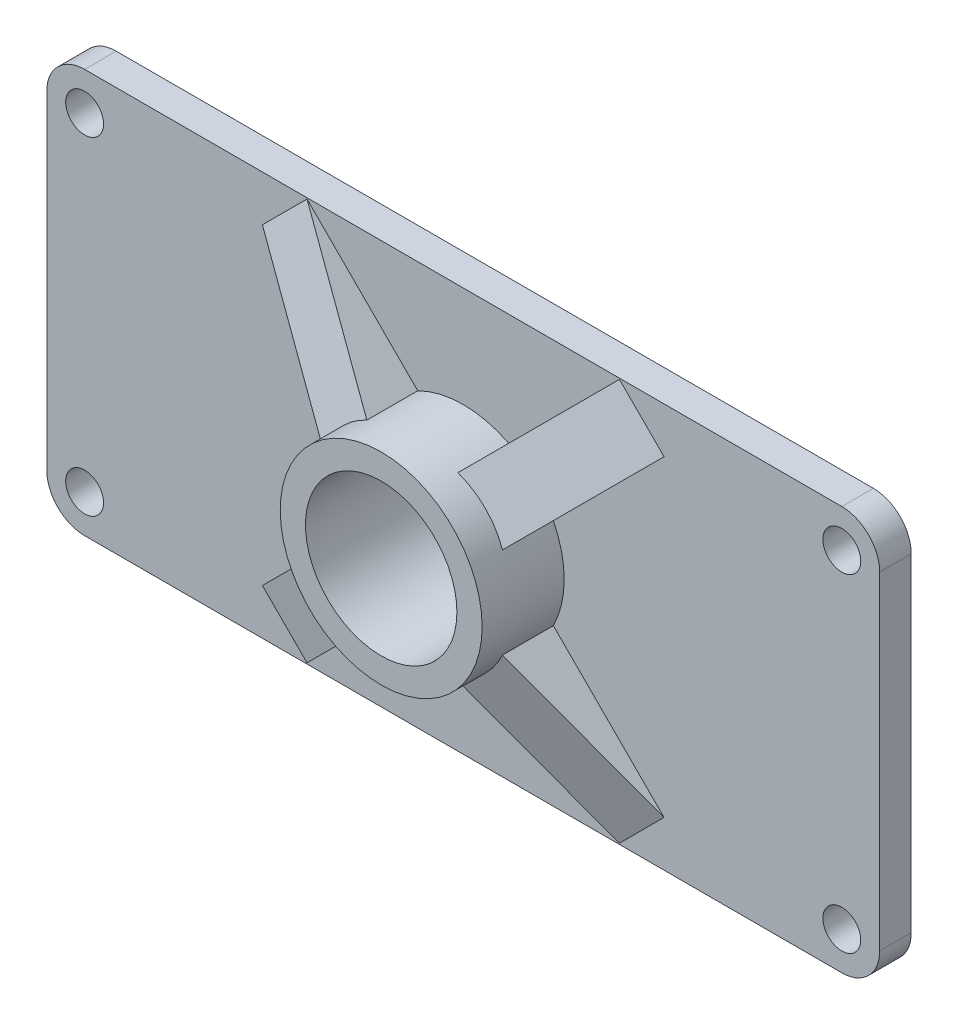
ISO-10303-21;
HEADER;
FILE_DESCRIPTION(('STEP AP214'),'2;1');
FILE_NAME('part.step','',(''),(''),'','','');
FILE_SCHEMA(('AUTOMOTIVE_DESIGN { 1 0 10303 214 1 1 1 1 }'));
ENDSEC;
DATA;
#1=APPLICATION_CONTEXT('core data for automotive mechanical design processes');
#2=APPLICATION_PROTOCOL_DEFINITION('international standard','automotive_design',2000,#1);
#3=PRODUCT_CONTEXT('',#1,'mechanical');
#4=PRODUCT('Part','Part','',(#3));
#5=PRODUCT_RELATED_PRODUCT_CATEGORY('part','',(#4));
#6=PRODUCT_DEFINITION_FORMATION('','',#4);
#7=PRODUCT_DEFINITION_CONTEXT('part definition',#1,'design');
#8=PRODUCT_DEFINITION('design','',#6,#7);
#9=PRODUCT_DEFINITION_SHAPE('','',#8);
#10=(LENGTH_UNIT() NAMED_UNIT(*) SI_UNIT(.MILLI.,.METRE.));
#11=(NAMED_UNIT(*) PLANE_ANGLE_UNIT() SI_UNIT($,.RADIAN.));
#12=(NAMED_UNIT(*) SI_UNIT($,.STERADIAN.) SOLID_ANGLE_UNIT());
#13=UNCERTAINTY_MEASURE_WITH_UNIT(LENGTH_MEASURE(1.E-05),#10,'distance_accuracy_value','');
#14=(GEOMETRIC_REPRESENTATION_CONTEXT(3) GLOBAL_UNCERTAINTY_ASSIGNED_CONTEXT((#13)) GLOBAL_UNIT_ASSIGNED_CONTEXT((#10,
#11,#12)) REPRESENTATION_CONTEXT('',''));
#15=CARTESIAN_POINT('',(0.,0.,0.));
#16=DIRECTION('',(0.,0.,1.));
#17=DIRECTION('',(1.,0.,0.));
#18=AXIS2_PLACEMENT_3D('',#15,#16,#17);
#19=CARTESIAN_POINT('',(-60.,-26.,5.));
#20=DIRECTION('',(0.,0.,1.));
#21=DIRECTION('',(1.,0.,0.));
#22=AXIS2_PLACEMENT_3D('',#19,#20,#21);
#23=PLANE('',#22);
#24=DIRECTION('',(0.70710678118655,-0.707106781186545,0.));
#25=VECTOR('',#24,1.);
#26=CARTESIAN_POINT('',(-13.4644660940675,20.5355339059328,5.));
#27=LINE('',#26,#25);
#28=CARTESIAN_POINT('',(14.2826265360351,-7.21155872416955,5.));
#29=VERTEX_POINT('',#28);
#30=CARTESIAN_POINT('',(31.8267955992102,-24.7557277873445,4.99999999999999));
#31=VERTEX_POINT('',#30);
#32=EDGE_CURVE('E225',#29,#31,#27,.T.);
#33=ORIENTED_EDGE('',*,*,#32,.T.);
#34=DIRECTION('',(-0.707106781186545,-0.70710678118655,0.));
#35=VECTOR('',#34,1.);
#36=CARTESIAN_POINT('',(-14.7087383067224,-71.2912616932773,5.));
#37=LINE('',#36,#35);
#38=CARTESIAN_POINT('',(24.7557277873447,-31.82679559921,5.));
#39=VERTEX_POINT('',#38);
#40=EDGE_CURVE('E228',#39,#31,#37,.F.);
#41=ORIENTED_EDGE('',*,*,#40,.F.);
#42=DIRECTION('',(0.70710678118655,-0.707106781186545,0.));
#43=VECTOR('',#42,1.);
#44=CARTESIAN_POINT('',(-20.5355339059329,13.4644660940673,5.));
#45=LINE('',#44,#43);
#46=CARTESIAN_POINT('',(7.21155872416964,-14.2826265360351,5.));
#47=VERTEX_POINT('',#46);
#48=EDGE_CURVE('E226',#47,#39,#45,.T.);
#49=ORIENTED_EDGE('',*,*,#48,.F.);
#50=CARTESIAN_POINT('',(0.,0.,5.));
#51=DIRECTION('',(0.,0.,1.));
#52=DIRECTION('',(1.,0.,0.));
#53=AXIS2_PLACEMENT_3D('',#50,#51,#52);
#54=CIRCLE('',#53,16.);
#55=CARTESIAN_POINT('',(-7.21155872416961,-14.2826265360351,5.));
#56=VERTEX_POINT('',#55);
#57=EDGE_CURVE('E251',#56,#47,#54,.T.);
#58=ORIENTED_EDGE('',*,*,#57,.F.);
#59=DIRECTION('',(-0.707106781186548,-0.707106781186547,0.));
#60=VECTOR('',#59,1.);
#61=CARTESIAN_POINT('',(-39.4644660940673,-46.5355339059327,5.));
#62=LINE('',#61,#60);
#63=CARTESIAN_POINT('',(-24.7557277873445,-31.82679559921,5.00000000000001));
#64=VERTEX_POINT('',#63);
#65=EDGE_CURVE('E237',#56,#64,#62,.T.);
#66=ORIENTED_EDGE('',*,*,#65,.T.);
#67=DIRECTION('',(-0.707106781186547,0.707106781186548,0.));
#68=VECTOR('',#67,1.);
#69=CARTESIAN_POINT('',(-45.2912616932773,-11.2912616932773,5.));
#70=LINE('',#69,#68);
#71=CARTESIAN_POINT('',(-31.82679559921,-24.7557277873445,5.));
#72=VERTEX_POINT('',#71);
#73=EDGE_CURVE('E242',#72,#64,#70,.F.);
#74=ORIENTED_EDGE('',*,*,#73,.F.);
#75=DIRECTION('',(-0.707106781186548,-0.707106781186547,0.));
#76=VECTOR('',#75,1.);
#77=CARTESIAN_POINT('',(-46.5355339059328,-39.4644660940673,5.));
#78=LINE('',#77,#76);
#79=CARTESIAN_POINT('',(-14.2826265360351,-7.21155872416961,5.));
#80=VERTEX_POINT('',#79);
#81=EDGE_CURVE('E238',#80,#72,#78,.T.);
#82=ORIENTED_EDGE('',*,*,#81,.F.);
#83=CARTESIAN_POINT('',(-14.2826265360352,7.21155872416946,5.));
#84=VERTEX_POINT('',#83);
#85=EDGE_CURVE('E256',#84,#80,#54,.T.);
#86=ORIENTED_EDGE('',*,*,#85,.F.);
#87=DIRECTION('',(-0.707106781186555,0.70710678118654,0.));
#88=VECTOR('',#87,1.);
#89=CARTESIAN_POINT('',(-20.5355339059333,13.4644660940675,5.));
#90=LINE('',#89,#88);
#91=CARTESIAN_POINT('',(-31.8267955992102,24.7557277873442,5.00000000000001));
#92=VERTEX_POINT('',#91);
#93=EDGE_CURVE('E56',#84,#92,#90,.T.);
#94=ORIENTED_EDGE('',*,*,#93,.T.);
#95=DIRECTION('',(0.70710678118654,0.707106781186555,0.));
#96=VECTOR('',#95,1.);
#97=CARTESIAN_POINT('',(-71.291261693277,-14.7087383067233,5.));
#98=LINE('',#97,#96);
#99=CARTESIAN_POINT('',(-24.7557277873449,31.8267955992098,4.99999999999999));
#100=VERTEX_POINT('',#99);
#101=EDGE_CURVE('E53',#100,#92,#98,.F.);
#102=ORIENTED_EDGE('',*,*,#101,.F.);
#103=DIRECTION('',(-0.707106781186555,0.70710678118654,0.));
#104=VECTOR('',#103,1.);
#105=CARTESIAN_POINT('',(-13.4644660940679,20.535533905933,5.));
#106=LINE('',#105,#104);
#107=CARTESIAN_POINT('',(-7.21155872416975,14.282626536035,5.));
#108=VERTEX_POINT('',#107);
#109=EDGE_CURVE('E187',#108,#100,#106,.T.);
#110=ORIENTED_EDGE('',*,*,#109,.F.);
#111=CARTESIAN_POINT('',(7.2115587241696,14.2826265360351,5.));
#112=VERTEX_POINT('',#111);
#113=EDGE_CURVE('E670',#112,#108,#54,.T.);
#114=ORIENTED_EDGE('',*,*,#113,.F.);
#115=DIRECTION('',(0.707106781186548,0.707106781186547,0.));
#116=VECTOR('',#115,1.);
#117=CARTESIAN_POINT('',(-46.5355339059328,-39.4644660940673,5.));
#118=LINE('',#117,#116);
#119=CARTESIAN_POINT('',(24.7557277873446,31.8267955992101,4.99999999999999));
#120=VERTEX_POINT('',#119);
#121=EDGE_CURVE('E211',#112,#120,#118,.T.);
#122=ORIENTED_EDGE('',*,*,#121,.T.);
#123=DIRECTION('',(0.707106781186547,-0.707106781186548,0.));
#124=VECTOR('',#123,1.);
#125=CARTESIAN_POINT('',(11.2912616932773,45.2912616932773,5.));
#126=LINE('',#125,#124);
#127=CARTESIAN_POINT('',(31.82679559921,24.7557277873446,5.));
#128=VERTEX_POINT('',#127);
#129=EDGE_CURVE('E213',#128,#120,#126,.F.);
#130=ORIENTED_EDGE('',*,*,#129,.F.);
#131=DIRECTION('',(0.707106781186548,0.707106781186547,0.));
#132=VECTOR('',#131,1.);
#133=CARTESIAN_POINT('',(-39.4644660940673,-46.5355339059327,5.));
#134=LINE('',#133,#132);
#135=CARTESIAN_POINT('',(14.2826265360351,7.21155872416959,5.));
#136=VERTEX_POINT('',#135);
#137=EDGE_CURVE('E206',#136,#128,#134,.T.);
#138=ORIENTED_EDGE('',*,*,#137,.F.);
#139=EDGE_CURVE('E260',#29,#136,#54,.T.);
#140=ORIENTED_EDGE('',*,*,#139,.F.);
#141=EDGE_LOOP('',(#33,#41,#49,#58,#66,#74,#82,#86,#94,#102,#110,#114,#122,#130,#138,#140));
#142=FACE_BOUND('',#141,.T.);
#143=DIRECTION('',(1.,0.,0.));
#144=VECTOR('',#143,1.);
#145=CARTESIAN_POINT('',(-60.,-32.,5.));
#146=LINE('',#145,#144);
#147=CARTESIAN_POINT('',(-60.,-32.,5.));
#148=VERTEX_POINT('',#147);
#149=CARTESIAN_POINT('',(60.,-32.,5.));
#150=VERTEX_POINT('',#149);
#151=EDGE_CURVE('E289',#148,#150,#146,.T.);
#152=ORIENTED_EDGE('',*,*,#151,.T.);
#153=CARTESIAN_POINT('',(60.,-26.,5.));
#154=DIRECTION('',(0.,0.,1.));
#155=DIRECTION('',(1.,0.,0.));
#156=AXIS2_PLACEMENT_3D('',#153,#154,#155);
#157=CIRCLE('',#156,6.);
#158=CARTESIAN_POINT('',(66.,-26.,5.));
#159=VERTEX_POINT('',#158);
#160=EDGE_CURVE('E295',#150,#159,#157,.T.);
#161=ORIENTED_EDGE('',*,*,#160,.T.);
#162=DIRECTION('',(0.,1.,0.));
#163=VECTOR('',#162,1.);
#164=CARTESIAN_POINT('',(66.,-26.,5.));
#165=LINE('',#164,#163);
#166=CARTESIAN_POINT('',(66.,26.,5.));
#167=VERTEX_POINT('',#166);
#168=EDGE_CURVE('E294',#159,#167,#165,.T.);
#169=ORIENTED_EDGE('',*,*,#168,.T.);
#170=CARTESIAN_POINT('',(60.,26.,5.));
#171=DIRECTION('',(0.,0.,1.));
#172=DIRECTION('',(-1.,0.,0.));
#173=AXIS2_PLACEMENT_3D('',#170,#171,#172);
#174=CIRCLE('',#173,6.);
#175=CARTESIAN_POINT('',(60.,32.,5.));
#176=VERTEX_POINT('',#175);
#177=EDGE_CURVE('E296',#167,#176,#174,.T.);
#178=ORIENTED_EDGE('',*,*,#177,.T.);
#179=DIRECTION('',(-1.,0.,0.));
#180=VECTOR('',#179,1.);
#181=CARTESIAN_POINT('',(-60.,32.,5.));
#182=LINE('',#181,#180);
#183=CARTESIAN_POINT('',(-60.,32.,5.));
#184=VERTEX_POINT('',#183);
#185=EDGE_CURVE('E297',#176,#184,#182,.T.);
#186=ORIENTED_EDGE('',*,*,#185,.T.);
#187=CARTESIAN_POINT('',(-60.,26.,5.));
#188=DIRECTION('',(0.,0.,1.));
#189=DIRECTION('',(-1.,0.,0.));
#190=AXIS2_PLACEMENT_3D('',#187,#188,#189);
#191=CIRCLE('',#190,6.);
#192=CARTESIAN_POINT('',(-66.,26.,5.));
#193=VERTEX_POINT('',#192);
#194=EDGE_CURVE('E299',#184,#193,#191,.T.);
#195=ORIENTED_EDGE('',*,*,#194,.T.);
#196=DIRECTION('',(0.,-1.,0.));
#197=VECTOR('',#196,1.);
#198=CARTESIAN_POINT('',(-66.,-26.,5.));
#199=LINE('',#198,#197);
#200=CARTESIAN_POINT('',(-66.,-26.,5.));
#201=VERTEX_POINT('',#200);
#202=EDGE_CURVE('E305',#193,#201,#199,.T.);
#203=ORIENTED_EDGE('',*,*,#202,.T.);
#204=CARTESIAN_POINT('',(-60.,-26.,5.));
#205=DIRECTION('',(0.,0.,1.));
#206=DIRECTION('',(1.,0.,0.));
#207=AXIS2_PLACEMENT_3D('',#204,#205,#206);
#208=CIRCLE('',#207,6.);
#209=EDGE_CURVE('E287',#201,#148,#208,.T.);
#210=ORIENTED_EDGE('',*,*,#209,.T.);
#211=EDGE_LOOP('',(#152,#161,#169,#178,#186,#195,#203,#210));
#212=FACE_BOUND('',#211,.T.);
#213=CARTESIAN_POINT('',(-60.,-26.,5.));
#214=DIRECTION('',(0.,0.,1.));
#215=DIRECTION('',(1.,0.,0.));
#216=AXIS2_PLACEMENT_3D('',#213,#214,#215);
#217=CIRCLE('',#216,3.);
#218=CARTESIAN_POINT('',(-57.,-26.,5.));
#219=VERTEX_POINT('',#218);
#220=EDGE_CURVE('E265',#219,#219,#217,.T.);
#221=ORIENTED_EDGE('',*,*,#220,.F.);
#222=EDGE_LOOP('',(#221));
#223=FACE_BOUND('',#222,.T.);
#224=CARTESIAN_POINT('',(60.,26.,5.));
#225=DIRECTION('',(0.,0.,1.));
#226=DIRECTION('',(1.,0.,0.));
#227=AXIS2_PLACEMENT_3D('',#224,#225,#226);
#228=CIRCLE('',#227,3.);
#229=CARTESIAN_POINT('',(63.,26.,5.));
#230=VERTEX_POINT('',#229);
#231=EDGE_CURVE('E273',#230,#230,#228,.T.);
#232=ORIENTED_EDGE('',*,*,#231,.F.);
#233=EDGE_LOOP('',(#232));
#234=FACE_BOUND('',#233,.T.);
#235=CARTESIAN_POINT('',(-60.,26.,5.));
#236=DIRECTION('',(0.,0.,1.));
#237=DIRECTION('',(1.,0.,0.));
#238=AXIS2_PLACEMENT_3D('',#235,#236,#237);
#239=CIRCLE('',#238,3.);
#240=CARTESIAN_POINT('',(-57.,26.,5.));
#241=VERTEX_POINT('',#240);
#242=EDGE_CURVE('E278',#241,#241,#239,.T.);
#243=ORIENTED_EDGE('',*,*,#242,.F.);
#244=EDGE_LOOP('',(#243));
#245=FACE_BOUND('',#244,.T.);
#246=CARTESIAN_POINT('',(60.,-26.,5.));
#247=DIRECTION('',(0.,0.,1.));
#248=DIRECTION('',(1.,0.,0.));
#249=AXIS2_PLACEMENT_3D('',#246,#247,#248);
#250=CIRCLE('',#249,3.);
#251=CARTESIAN_POINT('',(63.,-26.,5.));
#252=VERTEX_POINT('',#251);
#253=EDGE_CURVE('E268',#252,#252,#250,.T.);
#254=ORIENTED_EDGE('',*,*,#253,.F.);
#255=EDGE_LOOP('',(#254));
#256=FACE_BOUND('',#255,.T.);
#257=ADVANCED_FACE('F39',(#142,#212,#223,#234,#245,#256),#23,.T.);
#258=CARTESIAN_POINT('',(-60.,-26.,0.));
#259=DIRECTION('',(0.,0.,1.));
#260=DIRECTION('',(1.,0.,0.));
#261=AXIS2_PLACEMENT_3D('',#258,#259,#260);
#262=PLANE('',#261);
#263=CARTESIAN_POINT('',(0.,0.,0.));
#264=DIRECTION('',(0.,0.,1.));
#265=DIRECTION('',(1.,0.,0.));
#266=AXIS2_PLACEMENT_3D('',#263,#264,#265);
#267=CIRCLE('',#266,12.);
#268=CARTESIAN_POINT('',(12.,0.,0.));
#269=VERTEX_POINT('',#268);
#270=EDGE_CURVE('E252',#269,#269,#267,.T.);
#271=ORIENTED_EDGE('',*,*,#270,.T.);
#272=EDGE_LOOP('',(#271));
#273=FACE_BOUND('',#272,.T.);
#274=CARTESIAN_POINT('',(60.,-26.,0.));
#275=DIRECTION('',(0.,0.,1.));
#276=DIRECTION('',(1.,0.,0.));
#277=AXIS2_PLACEMENT_3D('',#274,#275,#276);
#278=CIRCLE('',#277,6.);
#279=CARTESIAN_POINT('',(60.,-32.,0.));
#280=VERTEX_POINT('',#279);
#281=CARTESIAN_POINT('',(66.,-26.,0.));
#282=VERTEX_POINT('',#281);
#283=EDGE_CURVE('E310',#280,#282,#278,.T.);
#284=ORIENTED_EDGE('',*,*,#283,.F.);
#285=DIRECTION('',(1.,0.,0.));
#286=VECTOR('',#285,1.);
#287=CARTESIAN_POINT('',(-60.,-32.,0.));
#288=LINE('',#287,#286);
#289=CARTESIAN_POINT('',(-60.,-32.,0.));
#290=VERTEX_POINT('',#289);
#291=EDGE_CURVE('E307',#290,#280,#288,.T.);
#292=ORIENTED_EDGE('',*,*,#291,.F.);
#293=CARTESIAN_POINT('',(-60.,-26.,0.));
#294=DIRECTION('',(0.,0.,1.));
#295=DIRECTION('',(1.,0.,0.));
#296=AXIS2_PLACEMENT_3D('',#293,#294,#295);
#297=CIRCLE('',#296,6.);
#298=CARTESIAN_POINT('',(-66.,-26.,0.));
#299=VERTEX_POINT('',#298);
#300=EDGE_CURVE('E282',#299,#290,#297,.T.);
#301=ORIENTED_EDGE('',*,*,#300,.F.);
#302=DIRECTION('',(0.,-1.,0.));
#303=VECTOR('',#302,1.);
#304=CARTESIAN_POINT('',(-66.,-26.,0.));
#305=LINE('',#304,#303);
#306=CARTESIAN_POINT('',(-66.,26.,0.));
#307=VERTEX_POINT('',#306);
#308=EDGE_CURVE('E286',#307,#299,#305,.T.);
#309=ORIENTED_EDGE('',*,*,#308,.F.);
#310=CARTESIAN_POINT('',(-60.,26.,0.));
#311=DIRECTION('',(0.,0.,1.));
#312=DIRECTION('',(-1.,0.,0.));
#313=AXIS2_PLACEMENT_3D('',#310,#311,#312);
#314=CIRCLE('',#313,6.);
#315=CARTESIAN_POINT('',(-60.,32.,0.));
#316=VERTEX_POINT('',#315);
#317=EDGE_CURVE('E320',#316,#307,#314,.T.);
#318=ORIENTED_EDGE('',*,*,#317,.F.);
#319=DIRECTION('',(-1.,0.,0.));
#320=VECTOR('',#319,1.);
#321=CARTESIAN_POINT('',(-60.,32.,0.));
#322=LINE('',#321,#320);
#323=CARTESIAN_POINT('',(60.,32.,0.));
#324=VERTEX_POINT('',#323);
#325=EDGE_CURVE('E312',#324,#316,#322,.T.);
#326=ORIENTED_EDGE('',*,*,#325,.F.);
#327=CARTESIAN_POINT('',(60.,26.,0.));
#328=DIRECTION('',(0.,0.,1.));
#329=DIRECTION('',(-1.,0.,0.));
#330=AXIS2_PLACEMENT_3D('',#327,#328,#329);
#331=CIRCLE('',#330,6.);
#332=CARTESIAN_POINT('',(66.,26.,0.));
#333=VERTEX_POINT('',#332);
#334=EDGE_CURVE('E311',#333,#324,#331,.T.);
#335=ORIENTED_EDGE('',*,*,#334,.F.);
#336=DIRECTION('',(0.,1.,0.));
#337=VECTOR('',#336,1.);
#338=CARTESIAN_POINT('',(66.,-26.,0.));
#339=LINE('',#338,#337);
#340=EDGE_CURVE('E313',#282,#333,#339,.T.);
#341=ORIENTED_EDGE('',*,*,#340,.F.);
#342=EDGE_LOOP('',(#284,#292,#301,#309,#318,#326,#335,#341));
#343=FACE_BOUND('',#342,.T.);
#344=CARTESIAN_POINT('',(60.,26.,0.));
#345=DIRECTION('',(0.,0.,1.));
#346=DIRECTION('',(1.,0.,0.));
#347=AXIS2_PLACEMENT_3D('',#344,#345,#346);
#348=CIRCLE('',#347,3.);
#349=CARTESIAN_POINT('',(63.,26.,0.));
#350=VERTEX_POINT('',#349);
#351=EDGE_CURVE('E271',#350,#350,#348,.T.);
#352=ORIENTED_EDGE('',*,*,#351,.T.);
#353=EDGE_LOOP('',(#352));
#354=FACE_BOUND('',#353,.T.);
#355=CARTESIAN_POINT('',(60.,-26.,0.));
#356=DIRECTION('',(0.,0.,1.));
#357=DIRECTION('',(1.,0.,0.));
#358=AXIS2_PLACEMENT_3D('',#355,#356,#357);
#359=CIRCLE('',#358,3.);
#360=CARTESIAN_POINT('',(63.,-26.,0.));
#361=VERTEX_POINT('',#360);
#362=EDGE_CURVE('E264',#361,#361,#359,.T.);
#363=ORIENTED_EDGE('',*,*,#362,.T.);
#364=EDGE_LOOP('',(#363));
#365=FACE_BOUND('',#364,.T.);
#366=CARTESIAN_POINT('',(-60.,26.,0.));
#367=DIRECTION('',(0.,0.,1.));
#368=DIRECTION('',(1.,0.,0.));
#369=AXIS2_PLACEMENT_3D('',#366,#367,#368);
#370=CIRCLE('',#369,3.);
#371=CARTESIAN_POINT('',(-57.,26.,0.));
#372=VERTEX_POINT('',#371);
#373=EDGE_CURVE('E280',#372,#372,#370,.T.);
#374=ORIENTED_EDGE('',*,*,#373,.T.);
#375=EDGE_LOOP('',(#374));
#376=FACE_BOUND('',#375,.T.);
#377=CARTESIAN_POINT('',(-60.,-26.,0.));
#378=DIRECTION('',(0.,0.,1.));
#379=DIRECTION('',(1.,0.,0.));
#380=AXIS2_PLACEMENT_3D('',#377,#378,#379);
#381=CIRCLE('',#380,3.);
#382=CARTESIAN_POINT('',(-57.,-26.,0.));
#383=VERTEX_POINT('',#382);
#384=EDGE_CURVE('E261',#383,#383,#381,.T.);
#385=ORIENTED_EDGE('',*,*,#384,.T.);
#386=EDGE_LOOP('',(#385));
#387=FACE_BOUND('',#386,.T.);
#388=ADVANCED_FACE('F377',(#273,#343,#354,#365,#376,#387),#262,.F.);
#389=CARTESIAN_POINT('',(-60.,-26.,5.));
#390=DIRECTION('',(0.,0.,-1.));
#391=DIRECTION('',(-1.,0.,0.));
#392=AXIS2_PLACEMENT_3D('',#389,#390,#391);
#393=CYLINDRICAL_SURFACE('',#392,6.);
#394=ORIENTED_EDGE('',*,*,#300,.T.);
#395=DIRECTION('',(0.,0.,-1.));
#396=VECTOR('',#395,1.);
#397=CARTESIAN_POINT('',(-60.,-32.,5.));
#398=LINE('',#397,#396);
#399=EDGE_CURVE('E339',#148,#290,#398,.T.);
#400=ORIENTED_EDGE('',*,*,#399,.F.);
#401=ORIENTED_EDGE('',*,*,#209,.F.);
#402=DIRECTION('',(0.,0.,-1.));
#403=VECTOR('',#402,1.);
#404=CARTESIAN_POINT('',(-66.,-26.,5.));
#405=LINE('',#404,#403);
#406=EDGE_CURVE('E304',#201,#299,#405,.T.);
#407=ORIENTED_EDGE('',*,*,#406,.T.);
#408=EDGE_LOOP('',(#394,#400,#401,#407));
#409=FACE_BOUND('',#408,.T.);
#410=ADVANCED_FACE('F41',(#409),#393,.T.);
#411=CARTESIAN_POINT('',(-60.,-32.,5.));
#412=DIRECTION('',(0.,1.,0.));
#413=DIRECTION('',(0.,0.,1.));
#414=AXIS2_PLACEMENT_3D('',#411,#412,#413);
#415=PLANE('',#414);
#416=DIRECTION('',(0.,0.,-1.));
#417=VECTOR('',#416,1.);
#418=CARTESIAN_POINT('',(60.,-32.,5.));
#419=LINE('',#418,#417);
#420=EDGE_CURVE('E340',#150,#280,#419,.T.);
#421=ORIENTED_EDGE('',*,*,#420,.F.);
#422=ORIENTED_EDGE('',*,*,#151,.F.);
#423=ORIENTED_EDGE('',*,*,#399,.T.);
#424=ORIENTED_EDGE('',*,*,#291,.T.);
#425=EDGE_LOOP('',(#421,#422,#423,#424));
#426=FACE_BOUND('',#425,.T.);
#427=ADVANCED_FACE('F413',(#426),#415,.F.);
#428=CARTESIAN_POINT('',(60.,-26.,5.));
#429=DIRECTION('',(0.,0.,-1.));
#430=DIRECTION('',(-1.,0.,0.));
#431=AXIS2_PLACEMENT_3D('',#428,#429,#430);
#432=CYLINDRICAL_SURFACE('',#431,6.);
#433=ORIENTED_EDGE('',*,*,#283,.T.);
#434=DIRECTION('',(0.,0.,-1.));
#435=VECTOR('',#434,1.);
#436=CARTESIAN_POINT('',(66.,-26.,5.));
#437=LINE('',#436,#435);
#438=EDGE_CURVE('E331',#159,#282,#437,.T.);
#439=ORIENTED_EDGE('',*,*,#438,.F.);
#440=ORIENTED_EDGE('',*,*,#160,.F.);
#441=ORIENTED_EDGE('',*,*,#420,.T.);
#442=EDGE_LOOP('',(#433,#439,#440,#441));
#443=FACE_BOUND('',#442,.T.);
#444=ADVANCED_FACE('F409',(#443),#432,.T.);
#445=CARTESIAN_POINT('',(66.,-26.,5.));
#446=DIRECTION('',(-1.,0.,0.));
#447=DIRECTION('',(0.,0.,1.));
#448=AXIS2_PLACEMENT_3D('',#445,#446,#447);
#449=PLANE('',#448);
#450=ORIENTED_EDGE('',*,*,#340,.T.);
#451=DIRECTION('',(0.,0.,-1.));
#452=VECTOR('',#451,1.);
#453=CARTESIAN_POINT('',(66.,26.,5.));
#454=LINE('',#453,#452);
#455=EDGE_CURVE('E332',#167,#333,#454,.T.);
#456=ORIENTED_EDGE('',*,*,#455,.F.);
#457=ORIENTED_EDGE('',*,*,#168,.F.);
#458=ORIENTED_EDGE('',*,*,#438,.T.);
#459=EDGE_LOOP('',(#450,#456,#457,#458));
#460=FACE_BOUND('',#459,.T.);
#461=ADVANCED_FACE('F406',(#460),#449,.F.);
#462=CARTESIAN_POINT('',(60.,26.,5.));
#463=DIRECTION('',(0.,0.,-1.));
#464=DIRECTION('',(-1.,0.,0.));
#465=AXIS2_PLACEMENT_3D('',#462,#463,#464);
#466=CYLINDRICAL_SURFACE('',#465,6.);
#467=ORIENTED_EDGE('',*,*,#334,.T.);
#468=DIRECTION('',(0.,0.,-1.));
#469=VECTOR('',#468,1.);
#470=CARTESIAN_POINT('',(60.,32.,5.));
#471=LINE('',#470,#469);
#472=EDGE_CURVE('E327',#176,#324,#471,.T.);
#473=ORIENTED_EDGE('',*,*,#472,.F.);
#474=ORIENTED_EDGE('',*,*,#177,.F.);
#475=ORIENTED_EDGE('',*,*,#455,.T.);
#476=EDGE_LOOP('',(#467,#473,#474,#475));
#477=FACE_BOUND('',#476,.T.);
#478=ADVANCED_FACE('F405',(#477),#466,.T.);
#479=CARTESIAN_POINT('',(-60.,32.,5.));
#480=DIRECTION('',(0.,-1.,0.));
#481=DIRECTION('',(0.,0.,-1.));
#482=AXIS2_PLACEMENT_3D('',#479,#480,#481);
#483=PLANE('',#482);
#484=ORIENTED_EDGE('',*,*,#325,.T.);
#485=DIRECTION('',(0.,0.,-1.));
#486=VECTOR('',#485,1.);
#487=CARTESIAN_POINT('',(-60.,32.,5.));
#488=LINE('',#487,#486);
#489=EDGE_CURVE('E324',#184,#316,#488,.T.);
#490=ORIENTED_EDGE('',*,*,#489,.F.);
#491=ORIENTED_EDGE('',*,*,#185,.F.);
#492=ORIENTED_EDGE('',*,*,#472,.T.);
#493=EDGE_LOOP('',(#484,#490,#491,#492));
#494=FACE_BOUND('',#493,.T.);
#495=ADVANCED_FACE('F398',(#494),#483,.F.);
#496=CARTESIAN_POINT('',(-60.,26.,5.));
#497=DIRECTION('',(0.,0.,-1.));
#498=DIRECTION('',(-1.,0.,0.));
#499=AXIS2_PLACEMENT_3D('',#496,#497,#498);
#500=CYLINDRICAL_SURFACE('',#499,6.);
#501=ORIENTED_EDGE('',*,*,#317,.T.);
#502=DIRECTION('',(0.,0.,-1.));
#503=VECTOR('',#502,1.);
#504=CARTESIAN_POINT('',(-66.,26.,5.));
#505=LINE('',#504,#503);
#506=EDGE_CURVE('E325',#193,#307,#505,.T.);
#507=ORIENTED_EDGE('',*,*,#506,.F.);
#508=ORIENTED_EDGE('',*,*,#194,.F.);
#509=ORIENTED_EDGE('',*,*,#489,.T.);
#510=EDGE_LOOP('',(#501,#507,#508,#509));
#511=FACE_BOUND('',#510,.T.);
#512=ADVANCED_FACE('F393',(#511),#500,.T.);
#513=CARTESIAN_POINT('',(-66.,-26.,5.));
#514=DIRECTION('',(1.,0.,0.));
#515=DIRECTION('',(0.,0.,-1.));
#516=AXIS2_PLACEMENT_3D('',#513,#514,#515);
#517=PLANE('',#516);
#518=ORIENTED_EDGE('',*,*,#308,.T.);
#519=ORIENTED_EDGE('',*,*,#406,.F.);
#520=ORIENTED_EDGE('',*,*,#202,.F.);
#521=ORIENTED_EDGE('',*,*,#506,.T.);
#522=EDGE_LOOP('',(#518,#519,#520,#521));
#523=FACE_BOUND('',#522,.T.);
#524=ADVANCED_FACE('F391',(#523),#517,.F.);
#525=CARTESIAN_POINT('',(-60.,26.,5.));
#526=DIRECTION('',(0.,0.,-1.));
#527=DIRECTION('',(-1.,0.,0.));
#528=AXIS2_PLACEMENT_3D('',#525,#526,#527);
#529=CYLINDRICAL_SURFACE('',#528,3.);
#530=ORIENTED_EDGE('',*,*,#242,.T.);
#531=EDGE_LOOP('',(#530));
#532=FACE_BOUND('',#531,.T.);
#533=ORIENTED_EDGE('',*,*,#373,.F.);
#534=EDGE_LOOP('',(#533));
#535=FACE_BOUND('',#534,.T.);
#536=ADVANCED_FACE('F389',(#532,#535),#529,.F.);
#537=CARTESIAN_POINT('',(60.,26.,5.));
#538=DIRECTION('',(0.,0.,-1.));
#539=DIRECTION('',(-1.,0.,0.));
#540=AXIS2_PLACEMENT_3D('',#537,#538,#539);
#541=CYLINDRICAL_SURFACE('',#540,3.);
#542=ORIENTED_EDGE('',*,*,#231,.T.);
#543=EDGE_LOOP('',(#542));
#544=FACE_BOUND('',#543,.T.);
#545=ORIENTED_EDGE('',*,*,#351,.F.);
#546=EDGE_LOOP('',(#545));
#547=FACE_BOUND('',#546,.T.);
#548=ADVANCED_FACE('F468',(#544,#547),#541,.F.);
#549=CARTESIAN_POINT('',(60.,-26.,5.));
#550=DIRECTION('',(0.,0.,-1.));
#551=DIRECTION('',(-1.,0.,0.));
#552=AXIS2_PLACEMENT_3D('',#549,#550,#551);
#553=CYLINDRICAL_SURFACE('',#552,3.);
#554=ORIENTED_EDGE('',*,*,#253,.T.);
#555=EDGE_LOOP('',(#554));
#556=FACE_BOUND('',#555,.T.);
#557=ORIENTED_EDGE('',*,*,#362,.F.);
#558=EDGE_LOOP('',(#557));
#559=FACE_BOUND('',#558,.T.);
#560=ADVANCED_FACE('F460',(#556,#559),#553,.F.);
#561=CARTESIAN_POINT('',(-60.,-26.,5.));
#562=DIRECTION('',(0.,0.,-1.));
#563=DIRECTION('',(-1.,0.,0.));
#564=AXIS2_PLACEMENT_3D('',#561,#562,#563);
#565=CYLINDRICAL_SURFACE('',#564,3.);
#566=ORIENTED_EDGE('',*,*,#220,.T.);
#567=EDGE_LOOP('',(#566));
#568=FACE_BOUND('',#567,.T.);
#569=ORIENTED_EDGE('',*,*,#384,.F.);
#570=EDGE_LOOP('',(#569));
#571=FACE_BOUND('',#570,.T.);
#572=ADVANCED_FACE('F454',(#568,#571),#565,.F.);
#573=CARTESIAN_POINT('',(0.,0.,5.));
#574=DIRECTION('',(0.,0.,-1.));
#575=DIRECTION('',(-1.,0.,0.));
#576=AXIS2_PLACEMENT_3D('',#573,#574,#575);
#577=CYLINDRICAL_SURFACE('',#576,12.);
#578=ORIENTED_EDGE('',*,*,#270,.F.);
#579=EDGE_LOOP('',(#578));
#580=FACE_BOUND('',#579,.T.);
#581=CARTESIAN_POINT('',(0.,0.,18.));
#582=DIRECTION('',(0.,0.,1.));
#583=DIRECTION('',(1.,0.,0.));
#584=AXIS2_PLACEMENT_3D('',#581,#582,#583);
#585=CIRCLE('',#584,12.);
#586=CARTESIAN_POINT('',(12.,0.,18.));
#587=VERTEX_POINT('',#586);
#588=EDGE_CURVE('E247',#587,#587,#585,.T.);
#589=ORIENTED_EDGE('',*,*,#588,.T.);
#590=EDGE_LOOP('',(#589));
#591=FACE_BOUND('',#590,.T.);
#592=ADVANCED_FACE('F457',(#580,#591),#577,.F.);
#593=CARTESIAN_POINT('',(0.,0.,18.));
#594=DIRECTION('',(0.,0.,1.));
#595=DIRECTION('',(1.,0.,0.));
#596=AXIS2_PLACEMENT_3D('',#593,#594,#595);
#597=PLANE('',#596);
#598=ORIENTED_EDGE('',*,*,#588,.F.);
#599=EDGE_LOOP('',(#598));
#600=FACE_BOUND('',#599,.T.);
#601=CARTESIAN_POINT('',(0.,0.,18.));
#602=DIRECTION('',(0.,0.,1.));
#603=DIRECTION('',(1.,0.,0.));
#604=AXIS2_PLACEMENT_3D('',#601,#602,#603);
#605=CIRCLE('',#604,16.);
#606=CARTESIAN_POINT('',(16.,0.,18.));
#607=VERTEX_POINT('',#606);
#608=EDGE_CURVE('E249',#607,#607,#605,.T.);
#609=ORIENTED_EDGE('',*,*,#608,.T.);
#610=EDGE_LOOP('',(#609));
#611=FACE_BOUND('',#610,.T.);
#612=ADVANCED_FACE('F464',(#600,#611),#597,.T.);
#613=CARTESIAN_POINT('',(0.,0.,18.));
#614=DIRECTION('',(0.,0.,-1.));
#615=DIRECTION('',(-1.,0.,0.));
#616=AXIS2_PLACEMENT_3D('',#613,#614,#615);
#617=CYLINDRICAL_SURFACE('',#616,16.);
#618=CARTESIAN_POINT('',(0.,0.,18.));
#619=DIRECTION('',(-0.218508012224407,0.218508012224406,-0.951056516295156));
#620=DIRECTION('',(0.672498511963961,-0.672498511963957,-0.309016994374941));
#621=AXIS2_PLACEMENT_3D('',#618,#619,#620);
#622=ELLIPSE('',#621,16.8233955878122,16.);
#623=CARTESIAN_POINT('',(7.21155872416964,-14.282626536035,13.061648161682));
#624=VERTEX_POINT('',#623);
#625=CARTESIAN_POINT('',(14.2826265360351,-7.21155872416955,13.061648161682));
#626=VERTEX_POINT('',#625);
#627=EDGE_CURVE('E355',#624,#626,#622,.F.);
#628=ORIENTED_EDGE('',*,*,#627,.T.);
#629=DIRECTION('',(0.,0.,-1.));
#630=VECTOR('',#629,1.);
#631=CARTESIAN_POINT('',(14.2826265360351,-7.21155872416955,18.));
#632=LINE('',#631,#630);
#633=EDGE_CURVE('E349',#29,#626,#632,.F.);
#634=ORIENTED_EDGE('',*,*,#633,.F.);
#635=ORIENTED_EDGE('',*,*,#139,.T.);
#636=DIRECTION('',(0.,0.,-1.));
#637=VECTOR('',#636,1.);
#638=CARTESIAN_POINT('',(14.2826265360351,7.21155872416958,18.));
#639=LINE('',#638,#637);
#640=CARTESIAN_POINT('',(14.2826265360351,7.21155872416959,13.061648161682));
#641=VERTEX_POINT('',#640);
#642=EDGE_CURVE('E201',#136,#641,#639,.F.);
#643=ORIENTED_EDGE('',*,*,#642,.T.);
#644=CARTESIAN_POINT('',(0.,0.,18.));
#645=DIRECTION('',(-0.218508012224406,-0.218508012224406,-0.951056516295156));
#646=DIRECTION('',(0.672498511963959,0.672498511963959,-0.309016994374941));
#647=AXIS2_PLACEMENT_3D('',#644,#645,#646);
#648=ELLIPSE('',#647,16.8233955878122,16.);
#649=CARTESIAN_POINT('',(7.2115587241696,14.2826265360351,13.061648161682));
#650=VERTEX_POINT('',#649);
#651=EDGE_CURVE('E50',#641,#650,#648,.F.);
#652=ORIENTED_EDGE('',*,*,#651,.T.);
#653=DIRECTION('',(0.,0.,-1.));
#654=VECTOR('',#653,1.);
#655=CARTESIAN_POINT('',(7.2115587241696,14.2826265360351,18.));
#656=LINE('',#655,#654);
#657=EDGE_CURVE('E207',#112,#650,#656,.F.);
#658=ORIENTED_EDGE('',*,*,#657,.F.);
#659=ORIENTED_EDGE('',*,*,#113,.T.);
#660=DIRECTION('',(0.,0.,-1.));
#661=VECTOR('',#660,1.);
#662=CARTESIAN_POINT('',(-7.21155872416975,14.282626536035,18.));
#663=LINE('',#662,#661);
#664=CARTESIAN_POINT('',(-7.21155872416975,14.282626536035,13.061648161682));
#665=VERTEX_POINT('',#664);
#666=EDGE_CURVE('E179',#108,#665,#663,.F.);
#667=ORIENTED_EDGE('',*,*,#666,.T.);
#668=CARTESIAN_POINT('',(0.,0.,18.));
#669=DIRECTION('',(0.218508012224409,-0.218508012224404,-0.951056516295156));
#670=DIRECTION('',(-0.672498511963966,0.672498511963952,-0.309016994374941));
#671=AXIS2_PLACEMENT_3D('',#668,#669,#670);
#672=ELLIPSE('',#671,16.8233955878122,16.);
#673=CARTESIAN_POINT('',(-14.2826265360352,7.21155872416946,13.061648161682));
#674=VERTEX_POINT('',#673);
#675=EDGE_CURVE('E11',#665,#674,#672,.F.);
#676=ORIENTED_EDGE('',*,*,#675,.T.);
#677=DIRECTION('',(0.,0.,-1.));
#678=VECTOR('',#677,1.);
#679=CARTESIAN_POINT('',(-14.2826265360352,7.21155872416946,18.));
#680=LINE('',#679,#678);
#681=EDGE_CURVE('E177',#84,#674,#680,.F.);
#682=ORIENTED_EDGE('',*,*,#681,.F.);
#683=ORIENTED_EDGE('',*,*,#85,.T.);
#684=DIRECTION('',(0.,0.,-1.));
#685=VECTOR('',#684,1.);
#686=CARTESIAN_POINT('',(-14.2826265360351,-7.2115587241696,18.));
#687=LINE('',#686,#685);
#688=CARTESIAN_POINT('',(-14.2826265360351,-7.21155872416961,13.061648161682));
#689=VERTEX_POINT('',#688);
#690=EDGE_CURVE('E350',#80,#689,#687,.F.);
#691=ORIENTED_EDGE('',*,*,#690,.T.);
#692=CARTESIAN_POINT('',(0.,0.,18.));
#693=DIRECTION('',(0.218508012224406,0.218508012224406,-0.951056516295156));
#694=DIRECTION('',(-0.672498511963959,-0.672498511963959,-0.309016994374941));
#695=AXIS2_PLACEMENT_3D('',#692,#693,#694);
#696=ELLIPSE('',#695,16.8233955878122,16.);
#697=CARTESIAN_POINT('',(-7.21155872416961,-14.2826265360351,13.061648161682));
#698=VERTEX_POINT('',#697);
#699=EDGE_CURVE('E341',#689,#698,#696,.F.);
#700=ORIENTED_EDGE('',*,*,#699,.T.);
#701=DIRECTION('',(0.,0.,-1.));
#702=VECTOR('',#701,1.);
#703=CARTESIAN_POINT('',(-7.21155872416961,-14.2826265360351,18.));
#704=LINE('',#703,#702);
#705=EDGE_CURVE('E258',#56,#698,#704,.F.);
#706=ORIENTED_EDGE('',*,*,#705,.F.);
#707=ORIENTED_EDGE('',*,*,#57,.T.);
#708=DIRECTION('',(0.,0.,-1.));
#709=VECTOR('',#708,1.);
#710=CARTESIAN_POINT('',(7.21155872416964,-14.282626536035,18.));
#711=LINE('',#710,#709);
#712=EDGE_CURVE('E353',#47,#624,#711,.F.);
#713=ORIENTED_EDGE('',*,*,#712,.T.);
#714=EDGE_LOOP('',(#628,#634,#635,#643,#652,#658,#659,#667,#676,#682,#683,#691,#700,#706,#707,#713));
#715=FACE_BOUND('',#714,.T.);
#716=ORIENTED_EDGE('',*,*,#608,.F.);
#717=EDGE_LOOP('',(#716));
#718=FACE_BOUND('',#717,.T.);
#719=ADVANCED_FACE('F173',(#715,#718),#617,.T.);
#720=CARTESIAN_POINT('',(0.,0.,18.));
#721=DIRECTION('',(0.218508012224406,0.218508012224406,-0.951056516295156));
#722=DIRECTION('',(-0.672498511963959,-0.672498511963959,-0.309016994374941));
#723=AXIS2_PLACEMENT_3D('',#720,#721,#722);
#724=PLANE('',#723);
#725=DIRECTION('',(-0.672498511963959,-0.672498511963959,-0.309016994374941));
#726=VECTOR('',#725,1.);
#727=CARTESIAN_POINT('',(-3.53553390593275,3.53553390593273,18.));
#728=LINE('',#727,#726);
#729=EDGE_CURVE('E233',#689,#72,#728,.T.);
#730=ORIENTED_EDGE('',*,*,#729,.T.);
#731=ORIENTED_EDGE('',*,*,#73,.T.);
#732=DIRECTION('',(-0.672498511963959,-0.672498511963959,-0.309016994374941));
#733=VECTOR('',#732,1.);
#734=CARTESIAN_POINT('',(3.53553390593273,-3.53553390593275,18.));
#735=LINE('',#734,#733);
#736=EDGE_CURVE('E235',#698,#64,#735,.T.);
#737=ORIENTED_EDGE('',*,*,#736,.F.);
#738=ORIENTED_EDGE('',*,*,#699,.F.);
#739=EDGE_LOOP('',(#730,#731,#737,#738));
#740=FACE_BOUND('',#739,.T.);
#741=ADVANCED_FACE('F573',(#740),#724,.F.);
#742=CARTESIAN_POINT('',(-3.53553390593274,3.53553390593274,9.));
#743=DIRECTION('',(-0.707106781186547,0.707106781186548,0.));
#744=DIRECTION('',(-0.707106781186548,-0.707106781186547,0.));
#745=AXIS2_PLACEMENT_3D('',#742,#743,#744);
#746=PLANE('',#745);
#747=ORIENTED_EDGE('',*,*,#690,.F.);
#748=ORIENTED_EDGE('',*,*,#81,.T.);
#749=ORIENTED_EDGE('',*,*,#729,.F.);
#750=EDGE_LOOP('',(#747,#748,#749));
#751=FACE_BOUND('',#750,.T.);
#752=ADVANCED_FACE('F576',(#751),#746,.T.);
#753=CARTESIAN_POINT('',(3.53553390593274,-3.53553390593274,9.));
#754=DIRECTION('',(-0.707106781186547,0.707106781186548,0.));
#755=DIRECTION('',(-0.707106781186548,-0.707106781186547,0.));
#756=AXIS2_PLACEMENT_3D('',#753,#754,#755);
#757=PLANE('',#756);
#758=ORIENTED_EDGE('',*,*,#65,.F.);
#759=ORIENTED_EDGE('',*,*,#705,.T.);
#760=ORIENTED_EDGE('',*,*,#736,.T.);
#761=EDGE_LOOP('',(#758,#759,#760));
#762=FACE_BOUND('',#761,.T.);
#763=ADVANCED_FACE('F589',(#762),#757,.F.);
#764=CARTESIAN_POINT('',(0.,0.,18.));
#765=DIRECTION('',(-0.218508012224407,0.218508012224406,-0.951056516295156));
#766=DIRECTION('',(0.672498511963961,-0.672498511963956,-0.309016994374941));
#767=AXIS2_PLACEMENT_3D('',#764,#765,#766);
#768=PLANE('',#767);
#769=DIRECTION('',(0.672498511963961,-0.672498511963956,-0.309016994374941));
#770=VECTOR('',#769,1.);
#771=CARTESIAN_POINT('',(-3.53553390593272,-3.53553390593276,18.));
#772=LINE('',#771,#770);
#773=EDGE_CURVE('E218',#624,#39,#772,.T.);
#774=ORIENTED_EDGE('',*,*,#773,.T.);
#775=ORIENTED_EDGE('',*,*,#40,.T.);
#776=DIRECTION('',(0.672498511963961,-0.672498511963956,-0.309016994374941));
#777=VECTOR('',#776,1.);
#778=CARTESIAN_POINT('',(3.53553390593273,3.53553390593274,18.));
#779=LINE('',#778,#777);
#780=EDGE_CURVE('E217',#626,#31,#779,.T.);
#781=ORIENTED_EDGE('',*,*,#780,.F.);
#782=ORIENTED_EDGE('',*,*,#627,.F.);
#783=EDGE_LOOP('',(#774,#775,#781,#782));
#784=FACE_BOUND('',#783,.T.);
#785=ADVANCED_FACE('F600',(#784),#768,.F.);
#786=CARTESIAN_POINT('',(-3.53553390593273,-3.53553390593275,9.));
#787=DIRECTION('',(-0.707106781186545,-0.70710678118655,0.));
#788=DIRECTION('',(0.70710678118655,-0.707106781186545,0.));
#789=AXIS2_PLACEMENT_3D('',#786,#787,#788);
#790=PLANE('',#789);
#791=ORIENTED_EDGE('',*,*,#712,.F.);
#792=ORIENTED_EDGE('',*,*,#48,.T.);
#793=ORIENTED_EDGE('',*,*,#773,.F.);
#794=EDGE_LOOP('',(#791,#792,#793));
#795=FACE_BOUND('',#794,.T.);
#796=ADVANCED_FACE('F607',(#795),#790,.T.);
#797=CARTESIAN_POINT('',(3.53553390593273,3.53553390593275,9.));
#798=DIRECTION('',(-0.707106781186545,-0.70710678118655,0.));
#799=DIRECTION('',(0.70710678118655,-0.707106781186545,0.));
#800=AXIS2_PLACEMENT_3D('',#797,#798,#799);
#801=PLANE('',#800);
#802=ORIENTED_EDGE('',*,*,#32,.F.);
#803=ORIENTED_EDGE('',*,*,#633,.T.);
#804=ORIENTED_EDGE('',*,*,#780,.T.);
#805=EDGE_LOOP('',(#802,#803,#804));
#806=FACE_BOUND('',#805,.T.);
#807=ADVANCED_FACE('F614',(#806),#801,.F.);
#808=CARTESIAN_POINT('',(0.,0.,18.));
#809=DIRECTION('',(-0.218508012224406,-0.218508012224406,-0.951056516295156));
#810=DIRECTION('',(0.672498511963959,0.672498511963959,-0.309016994374941));
#811=AXIS2_PLACEMENT_3D('',#808,#809,#810);
#812=PLANE('',#811);
#813=DIRECTION('',(0.672498511963959,0.672498511963959,-0.309016994374941));
#814=VECTOR('',#813,1.);
#815=CARTESIAN_POINT('',(3.53553390593275,-3.53553390593273,18.));
#816=LINE('',#815,#814);
#817=EDGE_CURVE('E199',#641,#128,#816,.T.);
#818=ORIENTED_EDGE('',*,*,#817,.T.);
#819=ORIENTED_EDGE('',*,*,#129,.T.);
#820=DIRECTION('',(0.672498511963959,0.672498511963959,-0.309016994374941));
#821=VECTOR('',#820,1.);
#822=CARTESIAN_POINT('',(-3.53553390593273,3.53553390593275,18.));
#823=LINE('',#822,#821);
#824=EDGE_CURVE('E200',#650,#120,#823,.T.);
#825=ORIENTED_EDGE('',*,*,#824,.F.);
#826=ORIENTED_EDGE('',*,*,#651,.F.);
#827=EDGE_LOOP('',(#818,#819,#825,#826));
#828=FACE_BOUND('',#827,.T.);
#829=ADVANCED_FACE('F364',(#828),#812,.F.);
#830=CARTESIAN_POINT('',(-3.53553390593274,3.53553390593274,9.));
#831=DIRECTION('',(0.707106781186547,-0.707106781186548,0.));
#832=DIRECTION('',(0.707106781186548,0.707106781186547,0.));
#833=AXIS2_PLACEMENT_3D('',#830,#831,#832);
#834=PLANE('',#833);
#835=ORIENTED_EDGE('',*,*,#121,.F.);
#836=ORIENTED_EDGE('',*,*,#657,.T.);
#837=ORIENTED_EDGE('',*,*,#824,.T.);
#838=EDGE_LOOP('',(#835,#836,#837));
#839=FACE_BOUND('',#838,.T.);
#840=ADVANCED_FACE('F365',(#839),#834,.F.);
#841=CARTESIAN_POINT('',(3.53553390593274,-3.53553390593274,9.));
#842=DIRECTION('',(0.707106781186547,-0.707106781186548,0.));
#843=DIRECTION('',(0.707106781186548,0.707106781186547,0.));
#844=AXIS2_PLACEMENT_3D('',#841,#842,#843);
#845=PLANE('',#844);
#846=ORIENTED_EDGE('',*,*,#642,.F.);
#847=ORIENTED_EDGE('',*,*,#137,.T.);
#848=ORIENTED_EDGE('',*,*,#817,.F.);
#849=EDGE_LOOP('',(#846,#847,#848));
#850=FACE_BOUND('',#849,.T.);
#851=ADVANCED_FACE('F369',(#850),#845,.T.);
#852=CARTESIAN_POINT('',(0.,0.,18.));
#853=DIRECTION('',(0.218508012224409,-0.218508012224404,-0.951056516295156));
#854=DIRECTION('',(-0.672498511963966,0.672498511963952,-0.309016994374941));
#855=AXIS2_PLACEMENT_3D('',#852,#853,#854);
#856=PLANE('',#855);
#857=DIRECTION('',(-0.672498511963966,0.672498511963952,-0.309016994374941));
#858=VECTOR('',#857,1.);
#859=CARTESIAN_POINT('',(3.53553390593269,3.53553390593278,18.));
#860=LINE('',#859,#858);
#861=EDGE_CURVE('E192',#665,#100,#860,.T.);
#862=ORIENTED_EDGE('',*,*,#861,.T.);
#863=ORIENTED_EDGE('',*,*,#101,.T.);
#864=DIRECTION('',(-0.672498511963966,0.672498511963952,-0.309016994374941));
#865=VECTOR('',#864,1.);
#866=CARTESIAN_POINT('',(-3.53553390593271,-3.53553390593277,18.));
#867=LINE('',#866,#865);
#868=EDGE_CURVE('E190',#674,#92,#867,.T.);
#869=ORIENTED_EDGE('',*,*,#868,.F.);
#870=ORIENTED_EDGE('',*,*,#675,.F.);
#871=EDGE_LOOP('',(#862,#863,#869,#870));
#872=FACE_BOUND('',#871,.T.);
#873=ADVANCED_FACE('F189',(#872),#856,.F.);
#874=CARTESIAN_POINT('',(-3.5355339059327,-3.53553390593277,9.));
#875=DIRECTION('',(0.70710678118654,0.707106781186555,0.));
#876=DIRECTION('',(-0.707106781186555,0.70710678118654,0.));
#877=AXIS2_PLACEMENT_3D('',#874,#875,#876);
#878=PLANE('',#877);
#879=ORIENTED_EDGE('',*,*,#93,.F.);
#880=ORIENTED_EDGE('',*,*,#681,.T.);
#881=ORIENTED_EDGE('',*,*,#868,.T.);
#882=EDGE_LOOP('',(#879,#880,#881));
#883=FACE_BOUND('',#882,.T.);
#884=ADVANCED_FACE('F186',(#883),#878,.F.);
#885=CARTESIAN_POINT('',(3.5355339059327,3.53553390593278,9.));
#886=DIRECTION('',(0.70710678118654,0.707106781186555,0.));
#887=DIRECTION('',(-0.707106781186555,0.70710678118654,0.));
#888=AXIS2_PLACEMENT_3D('',#885,#886,#887);
#889=PLANE('',#888);
#890=ORIENTED_EDGE('',*,*,#666,.F.);
#891=ORIENTED_EDGE('',*,*,#109,.T.);
#892=ORIENTED_EDGE('',*,*,#861,.F.);
#893=EDGE_LOOP('',(#890,#891,#892));
#894=FACE_BOUND('',#893,.T.);
#895=ADVANCED_FACE('F653',(#894),#889,.T.);
#896=CLOSED_SHELL('',(#257,#388,#410,#427,#444,#461,#478,#495,#512,#524,#536,#548,#560,#572,
#592,#612,#719,#741,#752,#763,#785,#796,#807,#829,#840,#851,#873,#884,#895));
#897=MANIFOLD_SOLID_BREP('B2',#896);
#898=ADVANCED_BREP_SHAPE_REPRESENTATION('',(#18,#897),#14);
#899=SHAPE_DEFINITION_REPRESENTATION(#9,#898);
ENDSEC;
END-ISO-10303-21;
